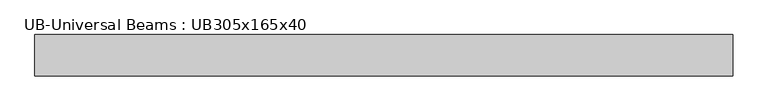
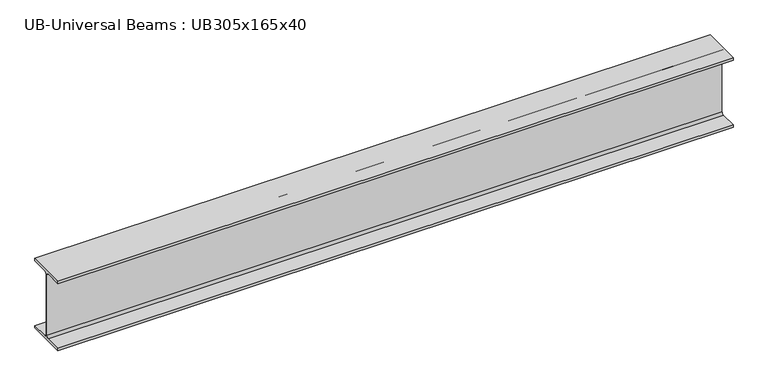
"""IFC4 building model written with IfcOpenShell, lengths in millimetres: beam geometry, UB-Universal Beams : UB305x165x40."""

from ifc_helpers import new_model, si_unit, point, frame, frame_2d, origin, place, context, project, spatial, polyline, circle_curve, trimmed, segment, composite_curve, outline, extrude, source, transform, mapped, element, save


def ub_universal_beams_ub305x165x40_82a0cad5(model_context):
    return source(origin(), model_context, "Body", "SweptSolid", [
        extrude(outline(composite_curve([segment(polyline([(82.5, -141.5), (82.5, -151.7), (-82.5, -151.7), (-82.5, -141.5), (-11.9, -141.5)]), True, "CONTINUOUS"), segment(trimmed(circle_curve(frame_2d((-11.9, -132.6)), 8.9), [point((-11.9, -141.5))], [point((-3.0, -132.6))], True, "CARTESIAN"), True, "CONTINUOUS"), segment(polyline([(-3.0, -132.6), (-3.0, 132.6)]), True, "CONTINUOUS"), segment(trimmed(circle_curve(frame_2d((-11.9, 132.6)), 8.9), [point((-3.0, 132.6))], [point((-11.9, 141.5))], True, "CARTESIAN"), True, "CONTINUOUS"), segment(polyline([(-11.9, 141.5), (-82.5, 141.5), (-82.5, 151.7), (82.5, 151.7), (82.5, 141.5), (11.9, 141.5)]), True, "CONTINUOUS"), segment(trimmed(circle_curve(frame_2d((11.9, 132.6)), 8.9), [point((11.9, 141.5))], [point((3.0, 132.6))], True, "CARTESIAN"), True, "CONTINUOUS"), segment(polyline([(3.0, 132.6), (3.0, -132.6)]), True, "CONTINUOUS"), segment(trimmed(circle_curve(frame_2d((11.9, -132.6)), 8.9), [point((3.0, -132.6))], [point((11.9, -141.5))], True, "CARTESIAN"), True, "CONTINUOUS"), segment(polyline([(11.9, -141.5), (82.5, -141.5)]), True, "CONTINUOUS")], self_intersect=False)), frame((-1387.3, 0.0, 0.0), z_axis=(1.0, 0.0, 0.0), x_axis=(0.0, 1.0, 0.0)), (0.0, 0.0, 1.0), 2792.1),
    ])


if __name__ == "__main__":
    model = new_model("IFC4")
    model_context = context("Model", 3, world=origin())
    ifc_project = project(units=[si_unit("LENGTHUNIT", "METRE", prefix="MILLI")], contexts=[model_context])
    site = spatial("IfcSite", under=ifc_project)
    building = spatial("IfcBuilding", under=site)
    placement = place(None, origin())
    ub_universal_beams_ub305x165x40_shape = ub_universal_beams_ub305x165x40_82a0cad5(model_context)
    element("IfcBeam", 1, ObjectType="UB-Universal Beams : UB305x165x40", at=placement, inside=building, context=model_context, shape_type="MappedRepresentation", body=[
        mapped(ub_universal_beams_ub305x165x40_shape, transform((0.0, 0.0, 0.0), x_axis=(1.0, 0.0, 0.0), y_axis=(0.0, 1.0, 0.0), z_axis=(0.0, 0.0, 1.0))),
    ])
    save(model, "model.ifc")

# Revit data of these elements
# Type "UB-Universal Beams : UB305x165x40"
#   Section Name Key = "UB305X165X40"
#   Width = 16.5 cm
#   Web Thickness = 0.6 cm
#   Web Fillet = 0.89 cm
#   Warping Constant = 164000.0 cm⁶
#   Torsional Moment of Inertia = 14.70 cm⁴
#   Section Area = 51.3 cm²
#   Plastic Modulus weak axis = 142.0 cm³
#   Plastic Modulus strong axis = 623.0 cm³
#   Nominal Weight = 40.2999 kgf/m
#   Moment of Inertia weak axis = 764.00 cm⁴
#   Moment of Inertia strong axis = 8503.00 cm⁴
#   Height = 30.34 cm
#   Flange Thickness = 1.02 cm
#   Elastic Modulus weak axis = 92.6 cm³
#   Elastic Modulus strong axis = 560.0 cm³
#   Centroid Vertical = 15.17 cm
#   Centroid Horizontal = 8.25 cm
#   Bolt Spacing = 9.0 cm
#   Length [instance default] = 1.5 m
#   Structural Material [instance default] = Metal - Steel 43-275
#   Type Comments = ""
#   Assembly Code = ""
# Element 1 (IfcBeam, "UB-Universal Beams : UB305x165x40")
#   Materials on its faces: "Metal - Steel 43-275"
# Materials
#   "Metal - Steel 43-275": class "Metal", colour RGB 247 247 247, transparency 0, Cost = 0
